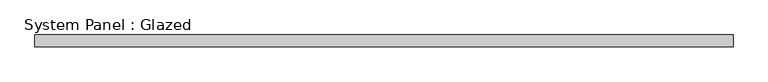
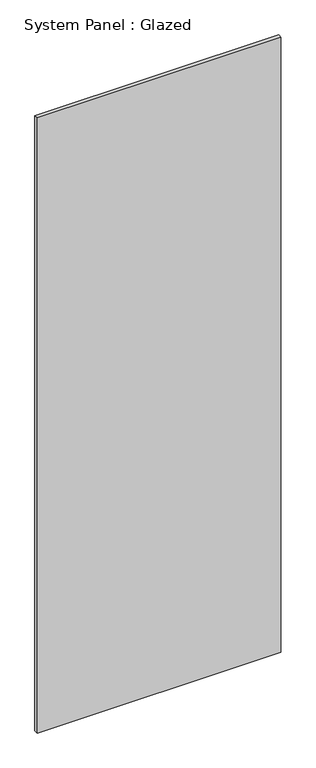
"""IFC4 building model written with IfcOpenShell, lengths in millimetres: plate geometry, System Panel : Glazed."""

from ifc_helpers import new_model, si_unit, origin, origin_with_axes, place, context, project, spatial, polyline, outline, extrude, source, transform, mapped, element, save


def system_panel_glazed_2e0a7f6c(model_context):
    return source(origin(), model_context, "Body", "SweptSolid", [
        extrude(outline(polyline([(749.3, 24.5), (-749.3, 24.5), (-749.3, 49.5), (749.3, 49.5), (749.3, 24.5)])), origin_with_axes(), (0.0, 0.0, 1.0), 4000.0),
    ])


if __name__ == "__main__":
    model = new_model("IFC4")
    model_context = context("Model", 3, world=origin())
    ifc_project = project(units=[si_unit("LENGTHUNIT", "METRE", prefix="MILLI")], contexts=[model_context])
    site = spatial("IfcSite", under=ifc_project)
    building = spatial("IfcBuilding", under=site)
    placement = place(None, origin())
    system_panel_glazed_shape = system_panel_glazed_2e0a7f6c(model_context)
    element("IfcPlate", 1, ObjectType="System Panel : Glazed", at=placement, inside=building, context=model_context, shape_type="MappedRepresentation", body=[
        mapped(system_panel_glazed_shape, transform((0.0, 0.0, 0.0), x_axis=(1.0, 0.0, 0.0), y_axis=(0.0, 1.0, 0.0), z_axis=(0.0, 0.0, 1.0))),
    ])
    save(model, "model.ifc")

# Revit data of these elements
# Type "System Panel : Glazed"
#   Keynote = "H11"
#   Construction Type Id = "GSP4R"
#   Analytic Construction = "1/8 in Pilkington single glazing"
#   Visual Light Transmittance = 0.9
#   Solar Heat Gain Coefficient = 0.86
#   Heat Transfer Coefficient (U) = 6.7069 W/(m²·K)
#   Define Thermal Properties by = 1
# Element 1 (IfcPlate, "System Panel : Glazed")
#   Materials on its faces: "Glass"
# Materials
#   "Glass": class "Glass", colour RGB 0 128 192, transparency 0.9, Description = "Soda Lime Glass", Cost = 0
